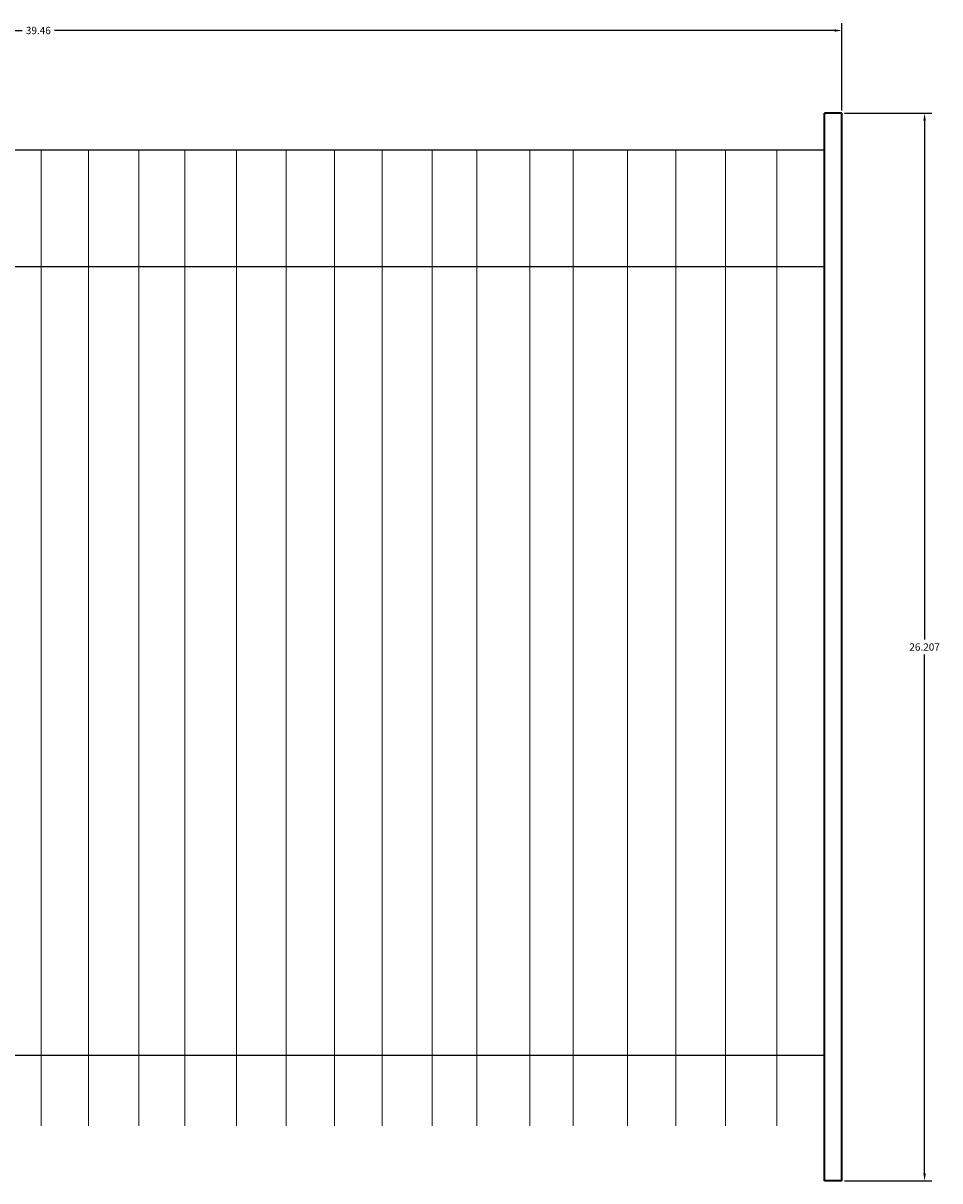
# Model space of a CAD drawing. Units: inches. Extents: x 756 to 915, y 488 to 695.
# Tile 22 of 25: x 885 to 908, y 594 to 622. Entities that reach past the tile are written whole.
import ezdxf

# ---------------------------------------------------------------- set-up
doc = ezdxf.new("R2010")
doc.units = ezdxf.units.IN
doc.header["$MEASUREMENT"] = 0
for name, color, linetype, lineweight in [('L-FENC-PCKT', 7, 'Continuous', 18), ('L-FENC-POST', 7, 'Continuous', 35), ('L-FENC-RAIL', 7, 'Continuous', 25), ('M-DIMS', 2, 'Continuous', 18)]:
    doc.layers.add(name, color=color, linetype=linetype, lineweight=lineweight)
doc.styles.get("Standard").update_dxf_attribs({"font": 'arial.ttf'})
doc.dimstyles.get("Standard").update_dxf_attribs({"dimtxt": 0.18, "dimasz": 0.18, "dimexe": 0.18, "dimexo": 0.0625, "dimgap": 0.09, "dimtad": 0, "dimtih": 1, "dimtoh": 1, "dimdec": 0, "dimzin": 0, "dimdsep": 46, "dimlunit": 3, "dimtxsty": 'Standard', "dimcen": 0.09, "dimadec": 0, "dimazin": 0, "dimtfac": 1, "dimtdec": 0, "dimtofl": 0, "dimtmove": 0, "dimatfit": 3, "dimfxl": 1, "dimtolj": 1, "dimtzin": 0, "dimarcsym": 0})

# ---------------------------------------------------------------- blocks, each defined once
blk = doc.blocks.new('FENCE-POST-RIGHT')
for p, q in [((0, 26.207), (0, 0)), ((0, 26.207), (0.427, 26.207)), ((0.427, 26.207), (0.427, 0)), ((0, 0), (0.427, 0))]:
    blk.add_line(p, q)
blk = doc.blocks.new('*D44')
at = {"layer": 'Defpoints', "color": 0, "transparency": 16777216}
for p in [(905.412, 622.071), (865.954, 620.041), (905.412, 620.041)]:
    blk.add_point(p, dxfattribs=at)
at = {"layer": 'M-DIMS', "color": 0, "lineweight": -2, "transparency": 16777216}
for p, q in [((865.954, 620.104), (865.954, 622.251)), ((866.134, 622.071), (885.289, 622.071)), ((905.232, 622.071), (886.076, 622.071)), ((905.412, 620.104), (905.412, 622.251))]:
    blk.add_line(p, q, dxfattribs=at)
at = {"layer": 'M-DIMS', "color": 0, "transparency": 16777216}
for points in [[(866.134, 622.101), (866.134, 622.041), (865.954, 622.071)], [(905.232, 622.101), (905.232, 622.041), (905.412, 622.071)]]:
    blk.add_solid(points, dxfattribs=at)
at = {"layer": 'M-DIMS', "color": 0, "transparency": 16777216, "insert": (885.683, 622.071), "char_height": 0.18, "attachment_point": 5}
blk.add_mtext('\\A1;39.46', dxfattribs=at)
blk = doc.blocks.new('*D45')
at = {"layer": 'Defpoints', "color": 0, "transparency": 16777216}
for p in [(905.412, 620.041), (907.442, 620.041), (905.412, 593.835)]:
    blk.add_point(p, dxfattribs=at)
at = {"layer": 'M-DIMS', "color": 0, "lineweight": -2, "transparency": 16777216}
for p, q in [((905.474, 620.041), (907.622, 620.041)), ((907.442, 619.861), (907.442, 607.12)), ((907.442, 594.015), (907.442, 606.756)), ((905.474, 593.835), (907.622, 593.835))]:
    blk.add_line(p, q, dxfattribs=at)
at = {"layer": 'M-DIMS', "color": 0, "transparency": 16777216}
for points in [[(907.412, 619.861), (907.472, 619.861), (907.442, 620.041)], [(907.412, 594.015), (907.472, 594.015), (907.442, 593.835)]]:
    blk.add_solid(points, dxfattribs=at)
at = {"layer": 'M-DIMS', "color": 0, "transparency": 16777216, "insert": (907.442, 606.938), "char_height": 0.18, "attachment_point": 5}
blk.add_mtext('\\A1;26.207', dxfattribs=at)

msp = doc.modelspace()

# ---------------------------------------------------------------- linework, layer by layer
at = {"layer": 'L-FENC-PCKT'}
for p, q in [((885.7521, 619.1305), (885.7521, 595.1842)), ((886.9163, 619.1305), (886.9163, 595.1842)), ((888.1521, 619.1305), (888.1521, 595.1842)), ((889.2775, 619.1305), (889.2775, 595.1842)), ((890.552, 619.1305), (890.552, 595.1842)), ((891.7671, 619.1305), (891.7671, 595.1842)), ((892.9519, 619.1305), (892.9519, 595.1842)), ((894.1283, 619.1305), (894.1283, 595.1842)), ((895.3518, 619.1305), (895.3518, 595.1842)), ((896.4495, 619.1305), (896.4495, 595.1842)), ((897.7517, 619.1305), (897.7517, 595.1842)), ((898.8107, 619.1305), (898.8107, 595.1842)), ((900.1516, 619.1305), (900.1516, 595.1842)), ((901.3319, 619.1305), (901.3319, 595.1842)), ((902.5515, 619.1305), (902.5515, 595.1842)), ((903.8132, 619.1305), (903.8132, 595.1842))]:
    msp.add_line(p, q, dxfattribs=at)
at = {"layer": 'L-FENC-RAIL'}
for p, q in [((866.3803, 619.1401), (904.9851, 619.1401)), ((866.3803, 616.2757), (904.9851, 616.2757)), ((866.3803, 596.9163), (904.9851, 596.9163))]:
    msp.add_line(p, q, dxfattribs=at)

# ---------------------------------------------------------------- block references
at = {"layer": 'L-FENC-POST', "rotation": 180}
msp.add_blockref('FENCE-POST-RIGHT', (905.4119, 620.0415), dxfattribs=at)

# ---------------------------------------------------------------- dimensions: what is measured, and where the dimension line sits
at = {"layer": 'M-DIMS'}
dim = msp.add_linear_dim(base=(905.4118, 622.0715), p1=(865.9536, 620.0415), p2=(905.4118, 620.0415), dimstyle='Standard', override={"dimdec": 2, "dimlfac": 1, "dimrnd": 0, "dimzin": 0, "dimdsep": 46, "dimlunit": 2}, dxfattribs=at)
dim.commit()
dim.dimension.update_dxf_attribs({"geometry": '*D44', "text_midpoint": (885.6827, 622.0715)})
dim = msp.add_linear_dim(base=(907.4418, 620.0415), p1=(905.4118, 593.8347), p2=(905.4118, 620.0415), angle=90, dimstyle='Standard', override={"dimdec": 3, "dimlfac": 1, "dimrnd": 0, "dimzin": 0, "dimdsep": 46, "dimlunit": 2}, dxfattribs=at)
dim.commit()
dim.dimension.update_dxf_attribs({"geometry": '*D45', "text_midpoint": (907.4418, 606.9381)})

doc.saveas('drawing.dxf')
